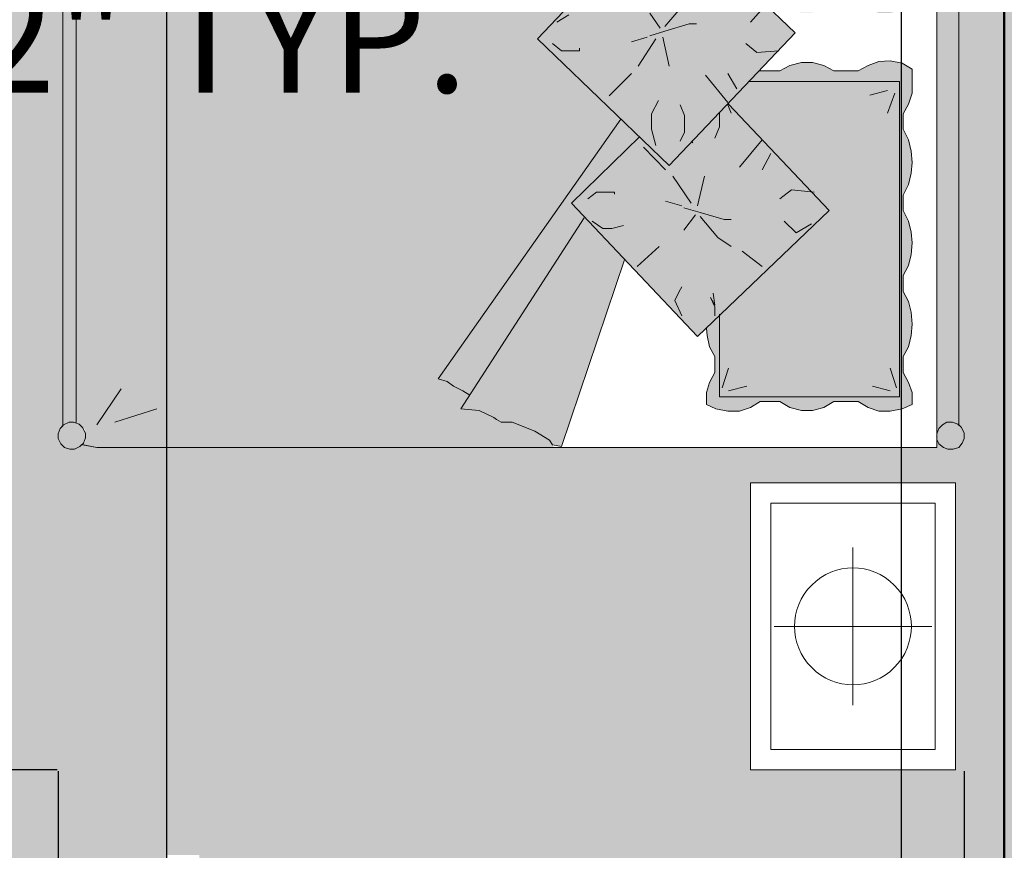
# Model space of a CAD drawing. Units: inches. Extents: x 528 to 2620, y -1066 to 798.
# Tile 28 of 41: x 1157 to 1211, y 620 to 665. Entities that reach past the tile are written whole.
import ezdxf

# ---------------------------------------------------------------- set-up
doc = ezdxf.new("R2010")
doc.units = ezdxf.units.IN
doc.header["$MEASUREMENT"] = 0
for name, color, linetype, lineweight in [('A-ANNO-DIMS', 2, 'Continuous', 18), ('A-FURN', 30, 'Continuous', 18), ('A-WALL', 7, 'Continuous', 50), ('A-WALL-PATT', 8, 'Continuous', 13)]:
    doc.layers.add(name, color=color, linetype=linetype, lineweight=lineweight)
doc.styles.get("Standard").update_dxf_attribs({"font": 'arial.ttf'})
doc.dimstyles.get("Standard").update_dxf_attribs({"dimtxt": 6, "dimasz": 2, "dimexe": 0.18, "dimexo": 0.0625, "dimgap": 0.09, "dimtad": 0, "dimtih": 1, "dimtoh": 1, "dimdec": 1, "dimzin": 0, "dimdsep": 46, "dimlunit": 3, "dimtxsty": 'Standard', "dimblk": 'ARCHTICK', "dimcen": 0.09, "dimadec": 0, "dimazin": 0, "dimtfac": 1, "dimtdec": 1, "dimtofl": 0, "dimtmove": 0, "dimatfit": 3, "dimfxl": 1, "dimtolj": 1, "dimtzin": 0, "dimarcsym": 0})

# ---------------------------------------------------------------- blocks, each defined once
blk = doc.blocks.new('d-bed-3')
at = {"color": 0, "linetype": 'ByBlock'}
for p, q in [((0.8389, 0.0078), (2.7305, 0.0078)), ((0.8409, 0.0078), (2.7305, 0.0078)), ((2.7234, -0.0077), (2.7284, 0.0056)), ((2.7284, 0.0056), (2.7365, 0.0144)), ((2.7305, 0.0078), (2.7365, 0.0144)), ((2.7365, 0.0144), (2.7505, 0.0211)), ((2.7365, 0.0144), (2.7505, 0.0211)), ((2.7505, 0.0211), (2.7636, 0.0211)), ((2.7505, 0.0211), (2.7636, 0.0211)), ((2.7636, 0.0211), (2.7746, 0.0166)), ((2.7636, 0.0211), (2.7746, 0.0166)), ((2.7746, 0.0166), (2.7857, 0.0078)), ((2.7746, 0.0166), (2.7857, 0.0078)), ((2.7857, 0.0078), (2.7897, -0.0054)), ((2.7857, 0.0078), (2.7897, -0.0054)), ((2.8714, -0.5), (2.8714, 0)), ((2.8714, 0), (3.5714, 0)), ((3.5714, 0), (3.5714, -0.5)), ((2.7234, -0.0209), (2.7234, -0.0077)), ((2.7305, -0.032), (2.7234, -0.0209)), ((2.7897, -0.0187), (2.7857, -0.0297)), ((2.7897, -0.0187), (2.7857, -0.0297)), ((2.7897, -0.0054), (2.7897, -0.0187)), ((2.7897, -0.0054), (2.7897, -0.0187)), ((2.7525, -0.0452), (0.8188, -0.0452)), ((2.7395, -0.0408), (2.7305, -0.032)), ((2.7525, -0.0452), (2.7395, -0.0408)), ((2.7656, -0.0452), (2.7525, -0.0452)), ((2.7766, -0.0408), (2.7656, -0.0452)), ((2.7766, -0.0408), (2.7656, -0.0452)), ((2.7656, -0.0452), (2.7857, -0.0452)), ((2.7857, -0.0452), (2.7656, -0.0452)), ((2.7857, -0.0297), (2.7766, -0.0408)), ((2.7857, -0.0297), (2.7766, -0.0408)), ((2.7857, -2.0939), (2.7857, -0.0452)), ((2.9214, -0.45), (2.9214, -0.05)), ((2.9214, -0.05), (3.5214, -0.05)), ((3.2214, -0.0576), (3.2214, -0.4424)), ((3.5214, -0.05), (3.5214, -0.45)), ((1.8489, -0.1302), (1.863, -0.1059)), ((1.863, -0.1059), (1.8951, -0.1059)), ((1.8951, -0.1059), (1.9222, -0.1059)), ((1.9222, -0.1059), (1.9483, -0.1148)), ((1.9483, -0.1148), (1.9724, -0.128)), ((2.0096, -0.128), (2.0357, -0.1148)), ((2.0357, -0.1148), (2.0628, -0.1082)), ((2.0628, -0.1082), (2.0909, -0.1059)), ((2.0909, -0.1059), (2.117, -0.1082)), ((2.117, -0.1082), (2.1441, -0.1148)), ((2.1441, -0.1148), (2.1702, -0.128)), ((2.2074, -0.128), (2.2335, -0.1148)), ((2.2335, -0.1148), (2.2606, -0.1082)), ((2.2606, -0.1082), (2.2867, -0.1059)), ((2.2867, -0.1059), (2.3148, -0.1082)), ((2.3148, -0.1082), (2.3419, -0.1148)), ((2.3419, -0.1148), (2.366, -0.128)), ((2.4052, -0.128), (2.4293, -0.1148)), ((2.4293, -0.1148), (2.4554, -0.1082)), ((2.4554, -0.1082), (2.4845, -0.1059)), ((2.4845, -0.1059), (2.5126, -0.1082)), ((2.5126, -0.1082), (2.5397, -0.1148)), ((2.5397, -0.1148), (2.5638, -0.128)), ((2.6029, -0.128), (2.627, -0.1148)), ((2.627, -0.1148), (2.6511, -0.1059)), ((2.6511, -0.1059), (2.6803, -0.1059)), ((2.6803, -0.1059), (2.6913, -0.1302)), ((1.8429, -0.159), (1.8489, -0.1302)), ((2.6622, -0.1369), (1.8931, -0.1369)), ((1.8931, -0.1369), (1.8931, -0.5046)), ((1.9724, -0.128), (2.0096, -0.128)), ((2.1702, -0.128), (2.2074, -0.128)), ((2.366, -0.128), (2.4052, -0.128)), ((2.5638, -0.128), (2.6029, -0.128)), ((2.6401, -0.1435), (2.5919, -0.159)), ((2.6622, -0.5753), (2.6622, -0.1369)), ((2.6913, -0.1302), (2.6973, -0.159)), ((1.8449, -0.1866), (1.8429, -0.159)), ((1.9152, -0.1656), (1.9263, -0.2087)), ((1.9222, -0.1479), (1.9704, -0.1656)), ((2.6471, -0.159), (2.6361, -0.202)), ((2.6973, -0.159), (2.6973, -0.1866)), ((1.854, -0.2131), (1.8449, -0.1866)), ((2.6973, -0.1866), (2.6883, -0.2131)), ((1.867, -0.2374), (1.854, -0.2131)), ((2.6883, -0.2131), (2.6732, -0.2374)), ((1.867, -0.297), (1.867, -0.2374)), ((2.6732, -0.2374), (2.6732, -0.297)), ((3.4138, -0.25), (3.029, -0.25)), ((1.854, -0.3213), (1.867, -0.297)), ((2.2074, -0.3081), (1.9483, -0.5532)), ((2.5146, -0.6294), (2.2074, -0.3081)), ((2.6732, -0.297), (2.6883, -0.3213)), ((1.8469, -0.3489), (1.854, -0.3213)), ((2.6883, -0.3213), (2.6953, -0.3489)), ((1.8469, -0.3754), (1.8469, -0.3489)), ((2.1632, -0.3445), (2.1572, -0.3997)), ((2.2405, -0.3511), (2.2626, -0.3887)), ((2.6953, -0.3489), (2.6953, -0.3754)), ((1.854, -0.4041), (1.8469, -0.3754)), ((2.6953, -0.3754), (2.6883, -0.4041)), ((1.4674, -0.7134), (1.7746, -0.3909)), ((1.7746, -0.3909), (2.0979, -0.6979)), ((1.867, -0.4284), (1.854, -0.4041)), ((2.1572, -0.3997), (2.1793, -0.4284)), ((2.2626, -0.3887), (2.2335, -0.4174)), ((2.6883, -0.4041), (2.6732, -0.4284)), ((1.8188, -0.4306), (1.8228, -0.4848)), ((1.867, -0.4781), (1.867, -0.4284)), ((2.6732, -0.4284), (2.6732, -0.4759)), ((2.0688, -0.4505), (2.109, -0.4715)), ((3.5214, -0.45), (2.9214, -0.45)), ((1.7194, -0.4737), (1.7485, -0.5002)), ((2.0357, -0.4715), (2.102, -0.5267)), ((2.3439, -0.4715), (2.3068, -0.5201)), ((2.6732, -0.4759), (2.6883, -0.5002)), ((1.8228, -0.4848), (1.8008, -0.5113)), ((2.6883, -0.5002), (2.6973, -0.5267)), ((3.5714, -0.5), (2.8714, -0.5)), ((2.6471, -0.5532), (2.6361, -0.5091)), ((2.6973, -0.5267), (2.6973, -0.5554)), ((1.9112, -0.5333), (1.874, -0.5554)), ((1.9704, -0.5466), (1.9503, -0.5554)), ((2.2295, -0.5643), (2.2295, -0.5466)), ((2.2736, -0.5797), (2.2957, -0.5466)), ((1.9443, -0.5554), (1.8781, -0.6096)), ((1.9684, -0.5753), (2.0036, -0.5753)), ((2.0036, -0.5753), (2.0317, -0.5864)), ((2.2124, -0.6228), (2.2295, -0.5643)), ((2.4604, -0.5753), (2.6622, -0.5753)), ((2.6401, -0.5687), (2.5919, -0.5532)), ((2.6973, -0.5554), (2.6913, -0.5841)), ((2.2224, -0.6228), (2.2736, -0.5797)), ((2.4383, -0.5864), (2.4092, -0.5908)), ((2.4423, -0.5864), (2.4202, -0.5974)), ((2.4202, -0.5974), (2.4383, -0.5864)), ((2.4644, -0.5864), (2.4423, -0.5864)), ((2.5397, -0.5996), (2.5126, -0.6051)), ((2.5638, -0.5864), (2.5397, -0.5996)), ((2.6029, -0.5864), (2.5638, -0.5864)), ((2.627, -0.5996), (2.6029, -0.5864)), ((2.6511, -0.6073), (2.627, -0.5996)), ((2.6913, -0.5841), (2.6803, -0.6073)), ((2.1963, -0.6294), (2.124, -0.6118)), ((2.2013, -0.6626), (2.2124, -0.6228)), ((2.5126, -0.6051), (2.4955, -0.6073)), ((2.6803, -0.6073), (2.6511, -0.6073)), ((1.7526, -0.6493), (1.7526, -0.6316)), ((2.0387, -0.6427), (2.0427, -0.6405)), ((2.1903, -0.6449), (2.124, -0.6891)), ((2.1903, -0.9365), (2.5146, -0.6294)), ((2.2556, -0.6626), (2.2184, -0.6338)), ((1.7596, -0.7089), (1.7084, -0.6648)), ((1.7706, -0.7089), (1.7526, -0.6493)), ((1.9765, -0.6604), (1.9503, -0.6714)), ((2.0166, -0.6604), (1.9765, -0.6604)), ((2.0387, -0.6714), (2.0166, -0.6604)), ((2.1963, -0.667), (2.1853, -0.7067)), ((2.4052, -0.6736), (2.3941, -0.667)), ((2.4644, -0.667), (2.4272, -0.6846)), ((2.4272, -0.6846), (2.4052, -0.6736)), ((1.7897, -1.0193), (1.4674, -0.7134)), ((1.7265, -0.7454), (1.7636, -0.72)), ((1.7817, -0.7454), (1.7706, -0.7089)), ((1.7857, -0.7134), (1.856, -0.6979)), ((2.0979, -0.6979), (1.7897, -1.0193)), ((2.0538, -0.7609), (2.109, -0.7067)), ((1.7897, -0.731), (1.856, -0.7741)), ((1.9724, -0.741), (1.9393, -0.7244)), ((2.0096, -0.741), (1.9724, -0.741)), ((2.0497, -0.731), (2.0096, -0.741)), ((2.3439, -0.7763), (2.2957, -0.7222)), ((1.7857, -0.752), (1.7967, -0.7896)), ((1.9283, -0.8448), (1.874, -0.7896)), ((2.1903, -0.9365), (2.0277, -0.7697)), ((2.618, -1.2611), (1.9855, -0.8161)), ((2.2515, -0.8382), (2.2445, -0.8094)), ((2.7827, -0.9607), (2.3278, -0.8072)), ((2.1632, -0.8757), (2.1632, -0.8315)), ((2.1632, -0.8315), (2.1682, -0.8315)), ((2.2515, -0.8602), (2.2515, -0.8382)), ((2.2335, -0.8856), (2.2515, -0.8602)), ((2.1793, -0.8967), (2.1632, -0.8757)), ((2.6913, -1.2059), (2.2254, -0.9055)), ((1.8188, -0.9166), (1.8118, -0.9166)), ((1.8188, -0.9607), (1.8188, -0.9166)), ((1.7485, -0.9718), (1.7305, -0.9431)), ((1.8008, -0.9828), (1.8188, -0.9607)), ((2.7786, -0.9828), (2.7676, -0.9895)), ((2.7827, -0.9607), (2.7786, -0.9828)), ((2.7676, -0.9895), (2.7455, -1.0259)), ((2.7455, -1.0259), (2.7234, -1.0811)), ((2.7234, -1.0811), (2.7234, -1.1076)), ((2.7124, -1.1253), (2.6953, -1.1617)), ((2.7174, -1.1187), (2.7124, -1.1253)), ((2.7234, -1.1076), (2.7174, -1.1187)), ((2.6953, -1.1617), (2.6913, -1.2059)), ((2.6582, -1.1838), (2.6471, -1.2015)), ((2.6361, -1.2236), (2.625, -1.2391)), ((2.6471, -1.2015), (2.6361, -1.2236)), ((2.625, -1.2391), (2.618, -1.2611)), ((2.7234, -2.0497), (2.6913, -1.947)), ((2.7305, -2.0939), (2.6421, -2.0342)), ((2.7857, -2.0939), (2.7783, -2.1299)), ((2.7786, -2.1281), (2.7857, -2.0939)), ((2.7365, -2.1281), (2.7284, -2.1369)), ((2.7505, -2.1215), (2.7365, -2.1281)), ((2.7616, -2.1215), (2.7505, -2.1215)), ((2.7746, -2.1259), (2.7616, -2.1215)), ((2.7827, -2.1347), (2.7746, -2.1259)), ((2.7783, -2.1299), (2.7827, -2.1347)), ((2.7827, -2.1347), (2.7897, -2.148)), ((2.7897, -2.148), (2.7827, -2.1347)), ((2.7264, -2.1436), (0.845, -2.1436)), ((2.7284, -2.1369), (2.7234, -2.1502)), ((2.7234, -2.1502), (2.7234, -2.1612)), ((2.7897, -2.159), (2.7857, -2.1723)), ((2.7857, -2.1723), (2.7897, -2.159)), ((2.7897, -2.148), (2.7897, -2.159)), ((2.7897, -2.159), (2.7897, -2.148)), ((2.7327, -2.1767), (0.8367, -2.1767)), ((0.8389, -2.1767), (2.7305, -2.1767)), ((2.7234, -2.1612), (2.7305, -2.1745)), ((2.7305, -2.1745), (2.7395, -2.1833)), ((2.7395, -2.1833), (2.7327, -2.1767)), ((2.7525, -2.1877), (2.7395, -2.1833)), ((2.7395, -2.1833), (2.7525, -2.1877)), ((2.7766, -2.1811), (2.7636, -2.1877)), ((2.7636, -2.1877), (2.7766, -2.1811)), ((2.7857, -2.1723), (2.7766, -2.1811)), ((2.7766, -2.1811), (2.7857, -2.1723)), ((2.7636, -2.1877), (2.7525, -2.1877)), ((2.7525, -2.1877), (2.7636, -2.1877))]:
    blk.add_line(p, q, dxfattribs=at)
at = {"color": 0, "linetype": 'ByBlock', "extrusion": (0, 0, -1)}
blk.add_ellipse((3.2214, -0.25), major_axis=(0.1007, 0.1007), ratio=1, dxfattribs=at)
blk = doc.blocks.new('_ArchTick')
at = {"color": 0, "linetype": 'ByBlock', "const_width": 0.15}
blk.add_lwpolyline([(-0.5, -0.5), (0.5, 0.5)], dxfattribs=at)
blk = doc.blocks.new('*D42')
at = {"layer": 'A-ANNO-DIMS', "color": 0, "lineweight": -2, "transparency": 16777216}
for p, q in [((1159.521, 703.64), (1147.464, 703.64)), ((1147.644, 703.64), (1147.644, 667.032)), ((1147.644, 624.039), (1147.644, 660.647)), ((1159.521, 624.039), (1147.464, 624.039))]:
    blk.add_line(p, q, dxfattribs=at)
at = {"layer": 'Defpoints', "color": 0, "transparency": 16777216}
for p in [(1159.584, 703.64), (1147.644, 624.039), (1159.584, 624.039)]:
    blk.add_point(p, dxfattribs=at)
at = {"layer": 'A-ANNO-DIMS', "color": 0, "lineweight": -2, "transparency": 16777216, "xscale": 2, "yscale": 2, "zscale": 2}
for p, rotation in [((1147.644, 703.64), 90), ((1147.644, 624.039), 270)]:
    blk.add_blockref('_ArchTick', p, dxfattribs=dict(at, rotation=rotation))
at = {"layer": 'A-ANNO-DIMS', "color": 0, "transparency": 16777216, "insert": (1147.644, 663.839), "char_height": 6, "attachment_point": 5}
blk.add_mtext('\\A1;BED 6\'-7 1/2" TYP.', dxfattribs=at)
blk = doc.blocks.new('*D43')
at = {"layer": 'A-ANNO-DIMS', "color": 0, "lineweight": -2, "transparency": 16777216}
for p, q in [((1159.584, 623.976), (1159.584, 611.919)), ((1208.815, 623.976), (1208.815, 611.919)), ((1159.584, 612.099), (1165.702, 612.099)), ((1208.815, 612.099), (1202.696, 612.099))]:
    blk.add_line(p, q, dxfattribs=at)
at = {"layer": 'Defpoints', "color": 0, "transparency": 16777216}
for p in [(1159.584, 624.039), (1208.815, 624.039), (1208.815, 612.099)]:
    blk.add_point(p, dxfattribs=at)
at = {"layer": 'A-ANNO-DIMS', "color": 0, "lineweight": -2, "transparency": 16777216, "xscale": 2, "yscale": 2, "zscale": 2, "rotation": 180}
blk.add_blockref('_ArchTick', (1159.584, 612.099), dxfattribs=at)
at = {"layer": 'A-ANNO-DIMS', "color": 0, "lineweight": -2, "transparency": 16777216, "xscale": 2, "yscale": 2, "zscale": 2}
blk.add_blockref('_ArchTick', (1208.815, 612.099), dxfattribs=at)
at = {"layer": 'A-ANNO-DIMS', "color": 0, "transparency": 16777216, "insert": (1184.199, 612.099), "char_height": 6, "attachment_point": 5}
blk.add_mtext('\\A1;4\'-1" TYP.', dxfattribs=at)
blk = doc.blocks.new('*D58')
at = {"layer": 'A-ANNO-DIMS', "color": 0, "lineweight": -2, "transparency": 16777216}
for p, q in [((1165.496, 577.985), (1165.496, 751.102)), ((1165.496, 750.922), (1177.395, 750.922)), ((1205.418, 750.922), (1193.52, 750.922)), ((1205.418, 577.985), (1205.418, 751.102))]:
    blk.add_line(p, q, dxfattribs=at)
at = {"layer": 'Defpoints', "color": 0, "transparency": 16777216}
for p in [(1205.418, 750.922), (1165.496, 577.922), (1205.418, 577.922)]:
    blk.add_point(p, dxfattribs=at)
at = {"layer": 'A-ANNO-DIMS', "color": 0, "lineweight": -2, "transparency": 16777216, "xscale": 2, "yscale": 2, "zscale": 2, "rotation": 180}
blk.add_blockref('_ArchTick', (1165.496, 750.922), dxfattribs=at)
at = {"layer": 'A-ANNO-DIMS', "color": 0, "lineweight": -2, "transparency": 16777216, "xscale": 2, "yscale": 2, "zscale": 2}
blk.add_blockref('_ArchTick', (1205.418, 750.922), dxfattribs=at)
at = {"layer": 'A-ANNO-DIMS', "color": 0, "transparency": 16777216, "insert": (1185.457, 750.922), "char_height": 6, "attachment_point": 5}
blk.add_mtext('\\A1;3\'-4"', dxfattribs=at)

msp = doc.modelspace()

# ---------------------------------------------------------------- hatches: boundary and pattern name
at = {"layer": 'A-WALL-PATT', "transparency": 33554521}
h = msp.add_hatch(color=256, dxfattribs=at)
h.dxf.hatch_style = 1
h.paths.add_polyline_path([(1065.996, 709.922), (1114.496, 709.922), (1114.496, 718.922), (1056.996, 718.922), (1056.996, 667.922), (1065.996, 667.922)])
h.paths.add_polyline_path([(1227.496, 718.922), (1162.496, 718.922), (1162.496, 709.922), (1210.996, 709.922), (1210.996, 577.922), (1205.418, 577.922), (1205.496, 573.422), (1210.996, 573.422), (1210.996, 567.422), (1215.496, 567.422), (1215.496, 669.422), (1267.996, 669.422), (1267.996, 675.922), (1263.496, 675.922), (1263.496, 673.922), (1215.496, 673.922), (1215.496, 709.922), (1227.496, 709.922)])
h.paths.add_polyline_path([(1344.996, 718.922), (1315.996, 718.922), (1315.996, 709.922), (1335.996, 709.922), (1335.996, 641.672), (1344.996, 641.672)])
h.paths.add_polyline_path([(1065.996, 619.922), (1056.996, 619.922), (1056.996, 561.422), (1065.996, 561.422), (1065.996, 573.422), (1160.996, 573.422), (1160.996, 569.422), (1165.496, 569.422), (1165.496, 577.922), (1065.996, 577.922)])
h.paths.add_polyline_path([(1215.996, 391.422), (1215.996, 400.422), (1206.996, 400.422), (1200.996, 400.422), (1200.996, 397.422), (1200.996, 391.422), (1206.996, 391.422), (1206.996, 268.922), (1251.996, 268.922), (1251.996, 277.922), (1215.996, 277.922), (1215.996, 359.767)])
h.paths.add_polyline_path([(1344.996, 395.922), (1335.996, 395.922), (1287.996, 395.922), (1287.996, 391.422), (1335.996, 391.422), (1335.996, 277.922), (1299.996, 277.922), (1299.996, 268.922), (1344.996, 268.922)])
h.paths.add_polyline_path([(1344.996, 593.672), (1335.996, 593.672), (1335.996, 525.422), (1215.496, 525.422), (1215.496, 527.172), (1210.996, 527.172), (1210.996, 520.922), (1335.996, 520.922), (1335.996, 443.922), (1344.996, 443.922)])
h.paths.add_polyline_path([(1065.996, 520.922), (1165.496, 520.922), (1165.496, 545.422), (1160.996, 545.422), (1160.996, 525.422), (1065.996, 525.422), (1065.996, 537.422), (1056.996, 537.422), (1056.996, 484.672), (1065.996, 484.672)])
h.paths.add_polyline_path([(1065.996, 436.672), (1056.996, 436.672), (1056.996, 391.422), (1085.496, 391.422), (1085.496, 400.422), (1065.996, 400.422)])
h.paths.add_polyline_path([(1152.996, 397.422), (1152.996, 400.422), (1133.496, 400.422), (1133.496, 391.422), (1152.996, 391.422)])
at = {"layer": 'A-WALL-PATT', "transparency": 33554536}
h = msp.add_hatch(color=256, dxfattribs=at)
h.dxf.hatch_style = 1
h.paths.add_polyline_path([(1335.996, 709.922), (1267.996, 709.922), (1267.996, 699.922), (1266.746, 699.922), (1266.746, 675.922), (1267.996, 675.922), (1267.996, 669.422), (1215.496, 669.422), (1215.496, 567.172), (1216.996, 567.172), (1256.996, 567.172), (1256.996, 565.422), (1256.958, 565.422, -0.401453), (1216.996, 527.172), (1215.496, 527.172), (1215.496, 525.422), (1335.996, 525.422)], flags=17)
h.paths.add_polyline_path([(1285.032, 635.927), (1285.229, 636.128), (1285.672, 636.263), (1286.206, 636.02), (1286.976, 636.084), (1332.983, 636.084), (1333.363, 636.222), (1333.82, 636.084), (1334.115, 635.714), (1334.115, 635.3), (1333.907, 634.86), (1333.82, 634.827), (1333.82, 592.738), (1333.967, 592.604), (1334.115, 592.291), (1334.115, 591.877), (1333.82, 591.507), (1333.363, 591.369), (1332.983, 591.507), (1332.638, 591.789), (1332.638, 591.507), (1286.976, 591.507), (1286.173, 591.672), (1286.066, 591.574), (1285.681, 591.37), (1285.229, 591.507), (1285.032, 591.709), (1284.834, 592.098), (1284.983, 592.537), (1285.13, 592.688), (1285.13, 634.948), (1284.983, 635.099), (1284.834, 635.537)], flags=16)
h.paths.add_polyline_path([(1285.032, 635.927), (1285.229, 636.128), (1285.672, 636.263), (1286.206, 636.02), (1286.976, 636.084), (1332.983, 636.084), (1333.363, 636.222), (1333.82, 636.084), (1334.115, 635.714), (1334.115, 635.3), (1333.967, 634.987), (1333.82, 634.853), (1333.82, 592.738), (1333.967, 592.604), (1334.115, 592.291), (1334.115, 591.877), (1333.82, 591.507), (1333.363, 591.369), (1332.983, 591.507), (1332.638, 591.789), (1332.638, 592.246), (1332.638, 635.345), (1332.638, 635.802), (1332.983, 636.084), (1312.232, 636.084), (1311.1, 635.479), (1310.632, 635.479), (1310.435, 635.233), (1309.943, 635.099), (1309.696, 634.987), (1309.056, 634.763), (1308.712, 634.607), (1308.318, 634.607), (1307.752, 634.36), (1307.112, 634.271), (1307.013, 634.114), (1306.767, 634.025), (1307.255, 633.283), (1306.866, 633.04), (1306.767, 632.884), (1306.373, 632.637), (1306.029, 632.548), (1305.536, 632.414), (1315.472, 618.494), (1316.321, 619.388), (1312.773, 622.858), (1319.616, 630.109), (1320.067, 629.676), (1320.109, 629.997), (1320.281, 630.601), (1320.527, 631.183), (1320.527, 632.011), (1320.256, 632.548), (1320.109, 633.13), (1320.06, 633.734), (1320.626, 634.025), (1321.216, 634.159), (1321.856, 634.114), (1322.447, 633.913), (1322.989, 633.622), (1324.096, 633.622), (1324.638, 633.913), (1325.229, 634.07), (1325.869, 634.07), (1326.435, 633.913), (1326.976, 633.622), (1328.355, 633.622), (1328.896, 633.913), (1329.487, 634.114), (1330.103, 634.159), (1330.693, 634.025), (1331.284, 633.734), (1331.235, 633.13), (1331.087, 632.548), (1330.792, 632.011), (1330.792, 631.183), (1331.038, 630.601), (1331.235, 629.997), (1331.284, 629.415), (1331.186, 628.788), (1331.038, 628.184), (1330.792, 627.602), (1330.792, 626.774), (1331.038, 626.193), (1331.235, 625.588), (1331.284, 625.007), (1331.186, 624.38), (1331.038, 623.776), (1330.792, 623.239), (1330.792, 622.366), (1331.038, 621.829), (1331.235, 621.247), (1331.284, 620.598), (1331.186, 619.972), (1331.038, 619.367), (1330.792, 618.83), (1330.792, 617.958), (1331.087, 617.421), (1331.235, 616.884), (1331.284, 616.235), (1331.284, 615.518), (1330.693, 615.272), (1330.103, 615.116), (1329.487, 615.116), (1328.896, 615.317), (1328.355, 615.653), (1326.976, 615.653), (1326.435, 615.317), (1325.869, 615.16), (1325.229, 615.16), (1324.638, 615.317), (1324.096, 615.653), (1323.242, 615.653), (1324.933, 614.042), (1322.978, 611.983), (1324.096, 611.983), (1324.638, 612.274), (1325.278, 612.43), (1325.869, 612.43), (1326.484, 612.274), (1327.026, 611.983), (1328.355, 611.983), (1328.896, 612.274), (1329.487, 612.475), (1330.103, 612.52), (1330.743, 612.386), (1331.284, 612.072), (1331.284, 611.356), (1331.284, 610.752), (1331.087, 610.17), (1330.792, 609.633), (1330.792, 608.805), (1331.087, 608.223), (1331.235, 607.619), (1331.284, 606.993), (1331.235, 606.411), (1331.087, 605.807), (1330.792, 605.225), (1330.792, 604.397), (1331.087, 603.815), (1331.235, 603.211), (1331.284, 602.629), (1331.235, 602.002), (1331.087, 601.398), (1330.792, 600.861), (1330.792, 599.988), (1331.087, 599.451), (1331.235, 598.87), (1331.284, 598.221), (1331.235, 597.594), (1331.087, 596.99), (1330.792, 596.453), (1330.792, 595.58), (1331.087, 595.043), (1331.284, 594.506), (1331.284, 593.857), (1330.743, 593.611), (1330.103, 593.477), (1329.487, 593.477), (1328.896, 593.678), (1328.355, 594.014), (1327.026, 594.014), (1326.484, 593.678), (1325.869, 593.521), (1325.278, 593.521), (1324.638, 593.678), (1324.096, 594.014), (1323.038, 594.014), (1322.496, 593.678), (1321.906, 593.477), (1321.266, 593.477), (1320.626, 593.611), (1320.109, 593.857), (1320.109, 594.506), (1320.281, 595.043), (1320.576, 595.58), (1320.576, 596.453), (1320.281, 596.99), (1320.158, 597.594), (1320.104, 598.015), (1319.616, 597.549), (1315.659, 601.729), (1312.232, 591.574), (1311.74, 591.664), (1311.592, 591.91), (1310.78, 592.402), (1309.549, 592.895), (1308.958, 592.895), (1308.712, 593.029), (1308.564, 593.141), (1307.752, 593.521), (1306.767, 593.611), (1307.248, 594.356), (1306.866, 594.595), (1306.373, 594.842), (1306.029, 595.088), (1305.536, 595.244), (1315.465, 609.354), (1310.927, 613.706), (1315.472, 618.494), (1305.536, 632.414), (1306.029, 632.548), (1306.373, 632.637), (1306.767, 632.884), (1306.866, 633.04), (1307.255, 633.283), (1306.767, 634.025), (1307.013, 634.114), (1307.112, 634.271), (1307.752, 634.36), (1308.318, 634.607), (1308.712, 634.607), (1309.056, 634.763), (1309.696, 634.987), (1309.943, 635.099), (1310.435, 635.233), (1310.632, 635.479), (1311.1, 635.479), (1312.232, 636.084), (1286.976, 636.084), (1286.216, 636.021), (1286.411, 635.444), (1286.213, 635.054), (1286.016, 634.853), (1285.869, 634.808), (1285.869, 592.839), (1286.153, 592.731), (1286.41, 592.188), (1286.231, 591.66), (1286.173, 591.672), (1286.066, 591.574), (1285.681, 591.37), (1285.229, 591.507), (1285.032, 591.709), (1284.834, 592.098), (1284.983, 592.537), (1285.13, 592.688), (1285.13, 634.948), (1284.983, 635.099), (1284.834, 635.537)], flags=0)
h.paths.add_polyline_path([(1322.501, 653.596), (1333.646, 653.596), (1333.646, 637.994), (1322.501, 637.994)], flags=16)
h.paths.add_polyline_path([(1323.616, 652.482), (1332.531, 652.482), (1332.531, 639.108), (1323.616, 639.108)], flags=0)
edge = h.paths.add_edge_path(flags=0)
edge.add_ellipse((1328.073, 645.795), major_axis=(2.245, 2.245), ratio=1, start_angle=405, end_angle=495, ccw=False)
edge.add_ellipse((1328.073, 645.795), major_axis=(2.245, 2.245), ratio=1, start_angle=675, end_angle=765, ccw=False)
edge.add_ellipse((1328.073, 645.795), major_axis=(2.245, 2.245), ratio=1, start_angle=585, end_angle=675, ccw=False)
edge.add_ellipse((1328.073, 645.795), major_axis=(2.245, 2.245), ratio=1, start_angle=495, end_angle=585, ccw=False)
h.paths.add_polyline_path([(1320.576, 628.386), (1320.33, 628.005), (1320.615, 628.548)], flags=0)
h.paths.add_polyline_path([(1317.893, 604.889), (1318.78, 604.643), (1319.764, 604.285), (1318.878, 604.531)], flags=0)
h.paths.add_polyline_path([(1320.33, 599.653), (1320.576, 599.25), (1320.576, 599.16)], flags=0)
h.paths.add_polyline_path([(1322.501, 589.597), (1333.646, 589.597), (1333.646, 573.995), (1322.501, 573.995)], flags=16)
h.paths.add_polyline_path([(1323.616, 588.482), (1332.531, 588.482), (1332.531, 575.109), (1323.616, 575.109)], flags=0)
edge = h.paths.add_edge_path(flags=0)
edge.add_ellipse((1328.073, 581.796), major_axis=(-2.245, 2.245), ratio=1, start_angle=-45, end_angle=45, ccw=False)
edge.add_ellipse((1328.073, 581.796), major_axis=(-2.245, 2.245), ratio=1, start_angle=-135, end_angle=-45, ccw=False)
edge.add_ellipse((1328.073, 581.796), major_axis=(-2.245, 2.245), ratio=1, start_angle=135, end_angle=-135, ccw=False)
edge.add_ellipse((1328.073, 581.796), major_axis=(-2.245, 2.245), ratio=1, start_angle=45, end_angle=135, ccw=False)
h.paths.add_polyline_path([(1264.746, 699.922), (1263.496, 699.922), (1263.496, 709.922), (1215.496, 709.922), (1215.496, 673.922), (1263.496, 673.922), (1263.496, 675.922), (1264.746, 675.922)], flags=16)
h.paths.add_polyline_path([(1162.192, 569.422), (1160.996, 569.422), (1160.996, 573.422), (1065.996, 573.422), (1065.996, 525.422), (1160.996, 525.422), (1160.996, 545.422), (1162.192, 545.422)])
h.paths.add_polyline_path([(1256.958, 565.422), (1256.996, 565.422), (1256.996, 567.172), (1216.996, 567.172), (1215.496, 567.172), (1215.496, 567.422), (1210.996, 567.422), (1210.996, 573.422), (1205.496, 573.422), (1205.418, 577.922), (1210.996, 577.922), (1210.996, 709.922), (1065.996, 709.922), (1065.996, 577.922), (1165.496, 577.922), (1165.496, 569.422), (1164.192, 569.422), (1164.192, 545.422), (1165.496, 545.422), (1165.496, 520.922), (1152.996, 520.922), (1152.996, 484.922), (1101.996, 484.922), (1101.996, 436.422), (1152.996, 436.422), (1152.996, 400.422), (1152.996, 391.422), (1200.996, 391.422), (1200.996, 400.422), (1206.996, 400.422), (1215.996, 400.422), (1215.996, 391.422), (1215.996, 277.922), (1335.996, 277.922), (1335.996, 391.422), (1287.996, 391.422), (1287.996, 395.922), (1335.996, 395.922), (1335.996, 443.922), (1335.996, 520.922), (1210.996, 520.922), (1210.996, 527.172), (1215.496, 527.172), (1216.996, 527.172, 0.401453)])
h.paths.add_polyline_path([(1167.246, 579.422), (1165.496, 579.422), (1165.496, 619.422), (1167.246, 619.422)], flags=16)
h.paths.add_polyline_path([(1227.97, 501.564), (1236.36, 502.031), (1236.36, 492.555), (1227.97, 493.021, -0.254069)], flags=16)
h.paths.add_polyline_path([(1243.336, 515.692, -0.254069), (1251.879, 515.692), (1252.345, 507.301), (1242.87, 507.301)], flags=16)
h.paths.add_polyline_path([(1239.185, 504.685), (1256.03, 504.685), (1256.03, 479.416), (1239.185, 479.416)], flags=16)
h.paths.add_polyline_path([(1227.97, 489.602), (1236.36, 490.068), (1236.36, 480.592), (1227.97, 481.058, -0.254069)], flags=16)
h.paths.add_polyline_path([(1197.201, 624.039), (1197.201, 639.641), (1208.345, 639.641), (1208.345, 624.039)], flags=16)
h.paths.add_polyline_path([(1198.315, 625.153), (1198.315, 638.526), (1207.231, 638.526), (1207.231, 625.153)], flags=0)
h.paths.add_polyline_path([(1258.855, 502.031), (1267.245, 501.564, -0.254069), (1267.245, 493.021), (1258.855, 492.555)], flags=16)
h.paths.add_polyline_path([(1271.589, 519.657), (1333.671, 519.657), (1333.671, 451.595), (1319.087, 451.595), (1319.087, 505.072), (1288.093, 505.072), (1284.447, 505.072, -0.883215), (1270.678, 514.188), (1270.678, 518.745, -0.414214)], flags=16)
h.paths.add_polyline_path([(1331.848, 517.834), (1331.848, 453.418), (1328.202, 453.418), (1328.202, 505.072), (1298.424, 505.072), (1298.424, 514.188), (1288.093, 514.188), (1288.093, 517.834)], flags=0)
h.paths.add_polyline_path([(1242.87, 476.8), (1252.345, 476.8), (1251.879, 468.409, -0.254069), (1243.336, 468.409)], flags=16)
h.paths.add_polyline_path([(1258.855, 490.068), (1267.245, 489.602, -0.254069), (1267.245, 481.058), (1258.855, 480.592)], flags=16)
h.paths.add_polyline_path([(1161.676, 641.551), (1160.873, 641.716), (1160.765, 641.618), (1160.38, 641.414), (1159.928, 641.551), (1159.731, 641.753), (1159.534, 642.142), (1159.682, 642.581), (1159.83, 642.732), (1159.83, 684.992), (1159.682, 685.143), (1159.534, 685.582), (1159.731, 685.971), (1159.928, 686.172), (1160.371, 686.307), (1160.905, 686.064), (1161.676, 686.128), (1207.682, 686.128), (1208.063, 686.266), (1208.519, 686.128), (1208.815, 685.758), (1208.815, 685.344), (1208.607, 684.904), (1208.519, 684.871), (1208.519, 642.782), (1208.667, 642.648), (1208.877, 642.201), (1208.716, 641.797), (1208.519, 641.551), (1208.063, 641.413), (1207.682, 641.551), (1207.338, 641.833), (1207.338, 641.551)], flags=16)
h.paths.add_polyline_path([(1186.931, 641.618), (1186.439, 641.708), (1186.291, 641.954), (1185.479, 642.446), (1184.248, 642.939), (1183.658, 642.939), (1183.411, 643.073), (1183.264, 643.185), (1182.451, 643.565), (1181.467, 643.655), (1181.948, 644.4), (1181.565, 644.639), (1181.073, 644.886), (1180.728, 645.132), (1180.236, 645.288), (1190.164, 659.398), (1185.627, 663.75), (1190.171, 668.538), (1180.236, 682.458), (1180.728, 682.592), (1181.073, 682.681), (1181.467, 682.928), (1181.565, 683.084), (1181.954, 683.327), (1181.467, 684.069), (1181.713, 684.158), (1181.811, 684.315), (1182.451, 684.404), (1183.018, 684.651), (1183.411, 684.651), (1183.756, 684.807), (1184.396, 685.031), (1184.642, 685.143), (1185.135, 685.277), (1185.331, 685.523), (1185.799, 685.523), (1186.931, 686.128), (1161.676, 686.128), (1160.915, 686.065), (1161.111, 685.488), (1160.913, 685.098), (1160.716, 684.897), (1160.568, 684.852), (1160.568, 642.883), (1160.853, 642.775), (1161.109, 642.232), (1160.931, 641.704), (1160.873, 641.716), (1160.765, 641.618), (1160.38, 641.414), (1159.928, 641.551), (1159.731, 641.753), (1159.534, 642.142), (1159.682, 642.581), (1159.83, 642.732), (1159.83, 684.992), (1159.682, 685.143), (1159.534, 685.582), (1159.731, 685.971), (1159.928, 686.172), (1160.371, 686.307), (1160.905, 686.064), (1161.676, 686.128), (1207.682, 686.128), (1208.063, 686.266), (1208.519, 686.128), (1208.815, 685.758), (1208.815, 685.344), (1208.667, 685.031), (1208.519, 684.897), (1208.519, 642.782), (1208.667, 642.648), (1208.877, 642.201), (1208.716, 641.797), (1208.519, 641.551), (1208.063, 641.413), (1207.682, 641.551), (1207.338, 641.833), (1207.338, 642.29), (1207.338, 685.389), (1207.338, 685.846), (1207.682, 686.128), (1186.931, 686.128), (1185.799, 685.523), (1185.331, 685.523), (1185.135, 685.277), (1184.642, 685.143), (1184.396, 685.031), (1183.756, 684.807), (1183.411, 684.651), (1183.018, 684.651), (1182.451, 684.404), (1181.811, 684.315), (1181.713, 684.158), (1181.467, 684.069), (1181.954, 683.327), (1181.565, 683.084), (1181.467, 682.928), (1181.073, 682.681), (1180.728, 682.592), (1180.236, 682.458), (1190.171, 668.538), (1191.021, 669.432), (1187.473, 672.902), (1194.316, 680.153), (1194.767, 679.72), (1194.808, 680.041), (1194.981, 680.645), (1195.227, 681.227), (1195.227, 682.055), (1194.956, 682.592), (1194.808, 683.174), (1194.759, 683.778), (1195.325, 684.069), (1195.916, 684.203), (1196.556, 684.158), (1197.147, 683.957), (1197.688, 683.666), (1198.796, 683.666), (1199.338, 683.957), (1199.928, 684.114), (1200.568, 684.114), (1201.135, 683.957), (1201.676, 683.666), (1203.055, 683.666), (1203.596, 683.957), (1204.187, 684.158), (1204.802, 684.203), (1205.393, 684.069), (1205.984, 683.778), (1205.935, 683.174), (1205.787, 682.592), (1205.491, 682.055), (1205.491, 681.227), (1205.738, 680.645), (1205.935, 680.041), (1205.984, 679.459), (1205.885, 678.832), (1205.738, 678.228), (1205.491, 677.646), (1205.491, 676.818), (1205.738, 676.237), (1205.935, 675.632), (1205.984, 675.051), (1205.885, 674.424), (1205.738, 673.82), (1205.491, 673.283), (1205.491, 672.41), (1205.738, 671.873), (1205.935, 671.291), (1205.984, 670.642), (1205.885, 670.016), (1205.738, 669.411), (1205.491, 668.874), (1205.491, 668.002), (1205.787, 667.465), (1205.935, 666.928), (1205.984, 666.279), (1205.984, 665.563), (1205.393, 665.316), (1204.802, 665.16), (1204.187, 665.16), (1203.596, 665.361), (1203.055, 665.697), (1201.676, 665.697), (1201.135, 665.361), (1200.568, 665.204), (1199.928, 665.204), (1199.338, 665.361), (1198.796, 665.697), (1197.942, 665.697), (1199.633, 664.086), (1197.678, 662.027), (1198.796, 662.027), (1199.338, 662.318), (1199.978, 662.474), (1200.568, 662.474), (1201.184, 662.318), (1201.725, 662.027), (1203.055, 662.027), (1203.596, 662.318), (1204.187, 662.519), (1204.802, 662.564), (1205.442, 662.43), (1205.984, 662.116), (1205.984, 661.4), (1205.984, 660.796), (1205.787, 660.214), (1205.491, 659.677), (1205.491, 658.849), (1205.787, 658.267), (1205.935, 657.663), (1205.984, 657.037), (1205.935, 656.455), (1205.787, 655.851), (1205.491, 655.269), (1205.491, 654.441), (1205.787, 653.859), (1205.935, 653.255), (1205.984, 652.673), (1205.935, 652.046), (1205.787, 651.442), (1205.491, 650.905), (1205.491, 650.032), (1205.787, 649.495), (1205.935, 648.914), (1205.984, 648.265), (1205.935, 647.638), (1205.787, 647.034), (1205.491, 646.497), (1205.491, 645.624), (1205.787, 645.087), (1205.984, 644.55), (1205.984, 643.901), (1205.442, 643.655), (1204.802, 643.521), (1204.187, 643.521), (1203.596, 643.722), (1203.055, 644.058), (1201.725, 644.058), (1201.184, 643.722), (1200.568, 643.565), (1199.978, 643.565), (1199.338, 643.722), (1198.796, 644.058), (1197.738, 644.058), (1197.196, 643.722), (1196.605, 643.521), (1195.965, 643.521), (1195.325, 643.655), (1194.808, 643.901), (1194.808, 644.55), (1194.981, 645.087), (1195.276, 645.624), (1195.276, 646.497), (1194.981, 647.034), (1194.858, 647.638), (1194.803, 648.059), (1194.316, 647.593), (1190.359, 651.773)], flags=16)
h.paths.add_polyline_path([(1195.276, 649.204), (1195.03, 649.697), (1195.276, 649.294)], flags=0)
h.paths.add_polyline_path([(1194.464, 654.329), (1193.578, 654.575), (1192.593, 654.933), (1193.479, 654.687)], flags=0)
h.paths.add_polyline_path([(1195.276, 678.43), (1195.03, 678.049), (1195.314, 678.592)], flags=0)
h.paths.add_polyline_path([(1197.201, 688.038), (1197.201, 703.64), (1208.345, 703.64), (1208.345, 688.038)], flags=16)
h.paths.add_polyline_path([(1198.315, 689.152), (1198.315, 702.526), (1207.231, 702.526), (1207.231, 689.152)], flags=0)
h.paths.add_polyline_path([(1217.099, 329.02), (1230.651, 329.02), (1230.651, 315.468), (1217.099, 315.468)], flags=16)
h.paths.add_polyline_path([(1223.875, 322.244), (1227.263, 322.244), (1227.263, 321.322, -0.414214), (1229.729, 318.856, -1), (1224.797, 318.856), (1223.875, 318.856)], flags=0)
h.paths.add_polyline_path([(1222.115, 325.632, -1), (1218.859, 325.632, -1)], flags=0)
h.paths.add_polyline_path([(1228.25, 325.632, -1), (1226.276, 325.632, -1)], flags=0)
h.paths.add_polyline_path([(1221.533, 318.856, -1), (1219.441, 318.856, -1)], flags=0)
h.paths.add_polyline_path([(1299.145, 293.732), (1299.145, 278.539), (1271.232, 278.539), (1271.232, 293.732)], flags=16)
h.paths.add_polyline_path([(1259.687, 292.213), (1270.624, 292.213, -1), (1270.624, 291.605), (1259.687, 291.605, -1)], flags=16)
h.paths.add_polyline_path([(1259.687, 291.301), (1270.624, 291.301, -1), (1270.624, 290.693), (1259.687, 290.693, -1)], flags=16)
h.paths.add_polyline_path([(1259.687, 290.389), (1270.624, 290.389, -1), (1270.624, 289.782), (1259.687, 289.782, -1)], flags=16)
h.paths.add_polyline_path([(1259.687, 289.478), (1270.624, 289.478, -1), (1270.624, 288.87), (1259.687, 288.87, -1)], flags=16)
h.paths.add_polyline_path([(1259.687, 288.566), (1270.624, 288.566, -1), (1270.624, 287.958), (1259.687, 287.958, -1)], flags=16)
h.paths.add_polyline_path([(1274.406, 292.381), (1283.251, 292.381, -0.414214), (1285.074, 290.558), (1285.074, 283.642, -0.414214), (1283.251, 281.819), (1277.723, 281.819), (1278.673, 280.869, -0.57735), (1279.382, 280.16), (1279.436, 280.106, -1), (1279.027, 279.696), (1278.972, 279.751, -0.57735), (1278.263, 280.46), (1276.904, 281.819), (1274.406, 281.819, -0.414214), (1272.583, 283.642), (1272.583, 290.558, -0.414214)], flags=0)
h.paths.add_polyline_path([(1259.687, 287.655), (1270.624, 287.655, -1), (1270.624, 287.047), (1259.687, 287.047, -1)], flags=16)
h.paths.add_polyline_path([(1259.687, 286.743), (1270.624, 286.743, -1), (1270.624, 286.135), (1259.687, 286.135, -1)], flags=16)
h.paths.add_polyline_path([(1259.687, 285.831), (1270.624, 285.831, -1), (1270.624, 285.224), (1259.687, 285.224, -1)], flags=16)
h.paths.add_polyline_path([(1259.687, 284.92), (1270.624, 284.92, -1), (1270.624, 284.312), (1259.687, 284.312, -1)], flags=16)
h.paths.add_polyline_path([(1259.687, 284.008), (1270.624, 284.008, -1), (1270.624, 283.401), (1259.687, 283.401, -1)], flags=16)
h.paths.add_polyline_path([(1287.823, 292.381), (1296.669, 292.381, -0.414214), (1298.492, 290.558), (1298.492, 283.642, -0.414214), (1296.669, 281.819), (1291.14, 281.819), (1292.09, 280.869, -0.57735), (1292.799, 280.16), (1292.854, 280.106, -1), (1292.445, 279.696), (1292.39, 279.751, -0.57735), (1291.681, 280.46), (1290.322, 281.819), (1287.823, 281.819, -0.414214), (1286, 283.642), (1286, 290.558, -0.414214)], flags=0)
h.paths.add_polyline_path([(1259.687, 283.097), (1270.624, 283.097, -1), (1270.624, 282.489), (1259.687, 282.489, -1)], flags=16)
h.paths.add_polyline_path([(1279.939, 287.607, -1), (1278.01, 287.607, -1)], flags=0)
h.paths.add_polyline_path([(1259.687, 282.185), (1270.624, 282.185, -1), (1270.624, 281.577), (1259.687, 281.577, -1)], flags=16)
h.paths.add_polyline_path([(1259.687, 281.273), (1270.624, 281.273, -1), (1270.624, 280.666), (1259.687, 280.666, -1)], flags=16)
h.paths.add_polyline_path([(1275.156, 284.169, -1), (1274.77, 284.169, -1)], flags=0)
h.paths.add_polyline_path([(1293.357, 287.607, -1), (1291.427, 287.607, -1)], flags=0)
h.paths.add_polyline_path([(1275.144, 280.503), (1276.335, 280.503, -5.828427), (1276.335, 280.117), (1275.144, 280.117, -1)], flags=0)
h.paths.add_polyline_path([(1288.574, 284.169, -1), (1288.188, 284.169, -1)], flags=0)
h.paths.add_polyline_path([(1281.31, 280.503), (1282.501, 280.503, -1), (1282.501, 280.117), (1281.31, 280.117, -5.828427)], flags=0)
h.paths.add_polyline_path([(1288.562, 280.503), (1289.752, 280.503, -5.828427), (1289.752, 280.117), (1288.562, 280.117, -1)], flags=0)
h.paths.add_polyline_path([(1294.727, 280.503), (1295.918, 280.503, -1), (1295.918, 280.117), (1294.727, 280.117, -5.828427)], flags=0)
h.paths.add_polyline_path([(1206.996, 391.422), (1200.996, 391.422), (1061.496, 391.422), (1061.496, 307.96), (1068.996, 307.96), (1068.996, 305.422), (1206.996, 305.422)])
at = {"layer": 'A-WALL-PATT', "transparency": 33554480}
h = msp.add_hatch(color=256, dxfattribs=at)
h.dxf.hatch_style = 1
h.paths.add_polyline_path([(1210.996, 709.922), (1065.996, 709.922), (1065.996, 577.922), (1165.496, 577.922), (1165.496, 579.422), (1165.496, 619.422), (1167.246, 619.422), (1167.246, 619.384, -0.401453), (1205.496, 579.422), (1205.496, 577.922), (1210.996, 577.922)])
h.paths.add_polyline_path([(1160.833, 686.058), (1160.905, 686.064), (1160.765, 686.128)], flags=16)
h.paths.add_polyline_path([(1160.931, 641.704), (1160.931, 641.707), (1160.928, 641.705)], flags=0)
h.paths.add_polyline_path([(1159.83, 684.992), (1159.584, 685.244), (1159.584, 685.82), (1160.016, 686.262), (1160.224, 686.262), (1159.928, 686.172), (1159.731, 685.971), (1159.584, 685.68), (1159.584, 685.434), (1159.682, 685.143), (1159.879, 684.942), (1160.175, 684.807), (1160.421, 684.807), (1160.716, 684.897), (1160.913, 685.098), (1161.111, 685.488), (1161.061, 685.635), (1161.061, 685.249), (1160.568, 684.746), (1160.568, 642.961), (1161.061, 642.514), (1161.061, 641.887), (1160.873, 641.716), (1161.676, 641.551), (1186.533, 641.551), (1186.291, 641.954), (1185.479, 642.446), (1184.248, 642.939), (1183.589, 642.939), (1183.264, 643.185), (1182.451, 643.565), (1181.467, 643.655), (1181.948, 644.4), (1181.565, 644.639), (1181.073, 644.886), (1180.728, 645.132), (1180.236, 645.288), (1190.164, 659.398), (1185.627, 663.75), (1190.171, 668.538), (1180.236, 682.458), (1180.728, 682.592), (1181.073, 682.681), (1181.467, 682.928), (1181.565, 683.084), (1181.954, 683.327), (1181.467, 684.069), (1181.713, 684.158), (1181.811, 684.315), (1182.451, 684.404), (1183.018, 684.651), (1183.411, 684.651), (1183.756, 684.807), (1184.396, 685.031), (1184.642, 685.143), (1185.135, 685.277), (1185.331, 685.523), (1185.799, 685.523), (1186.931, 686.128), (1207.682, 686.128), (1208.063, 686.266), (1208.631, 686.094), (1208.877, 685.478), (1208.607, 684.904), (1208.519, 684.871), (1208.519, 642.782), (1208.815, 642.514), (1208.815, 641.921), (1208.448, 641.462), (1207.792, 641.462), (1207.338, 641.833), (1207.338, 641.551), (1161.676, 641.551), (1160.928, 641.705), (1160.38, 641.414), (1159.816, 641.585), (1159.534, 642.142), (1159.722, 642.699), (1159.83, 642.756)], flags=16)
h.paths.add_polyline_path([(1159.83, 684.992), (1159.584, 685.244), (1159.584, 685.82), (1160.016, 686.262), (1160.224, 686.262), (1159.928, 686.172), (1159.731, 685.971), (1159.584, 685.68), (1159.584, 685.434), (1159.682, 685.143), (1159.83, 684.992), (1159.83, 642.732), (1159.682, 642.581), (1159.584, 642.29), (1159.584, 642.044), (1159.731, 641.753), (1160.016, 641.462), (1160.224, 641.462), (1159.816, 641.585), (1159.534, 642.142), (1159.682, 642.581), (1159.83, 642.732)], flags=0)
h.paths.add_polyline_path([(1207.682, 686.128), (1207.517, 686.128), (1207.488, 686.057)], flags=0)
h.paths.add_polyline_path([(1195.276, 648.712), (1195.287, 648.521), (1195.522, 648.746), (1195.522, 648.802), (1195.276, 649.204)], flags=0)
h.paths.add_polyline_path([(1194.767, 679.72), (1194.808, 680.041), (1194.981, 680.645), (1195.227, 681.227), (1195.227, 682.055), (1194.956, 682.592), (1194.808, 683.174), (1194.759, 683.778), (1195.325, 684.069), (1195.916, 684.203), (1196.556, 684.158), (1197.147, 683.957), (1197.688, 683.666), (1198.796, 683.666), (1199.338, 683.957), (1199.928, 684.114), (1200.568, 684.114), (1201.135, 683.957), (1201.676, 683.666), (1203.055, 683.666), (1203.596, 683.957), (1204.187, 684.158), (1204.802, 684.203), (1205.393, 684.069), (1205.984, 683.778), (1205.935, 683.174), (1205.787, 682.592), (1205.491, 682.055), (1205.491, 681.227), (1205.738, 680.645), (1205.935, 680.041), (1205.984, 679.459), (1205.885, 678.832), (1205.738, 678.228), (1205.491, 677.646), (1205.491, 676.818), (1205.738, 676.237), (1205.935, 675.632), (1205.984, 675.051), (1205.885, 674.424), (1205.738, 673.82), (1205.491, 673.283), (1205.491, 672.41), (1205.738, 671.873), (1205.935, 671.291), (1205.984, 670.642), (1205.885, 670.016), (1205.738, 669.411), (1205.491, 668.874), (1205.491, 668.002), (1205.787, 667.465), (1205.935, 666.928), (1205.984, 666.279), (1205.984, 665.563), (1205.393, 665.316), (1204.802, 665.16), (1204.187, 665.16), (1203.596, 665.361), (1203.055, 665.697), (1201.676, 665.697), (1201.135, 665.361), (1200.568, 665.204), (1199.928, 665.204), (1199.338, 665.361), (1198.796, 665.697), (1197.942, 665.697), (1199.633, 664.086), (1197.678, 662.027), (1198.796, 662.027), (1199.338, 662.318), (1199.978, 662.474), (1200.568, 662.474), (1201.184, 662.318), (1201.725, 662.027), (1203.055, 662.027), (1203.596, 662.318), (1204.187, 662.519), (1204.802, 662.564), (1205.442, 662.43), (1205.984, 662.116), (1205.984, 661.4), (1205.984, 660.796), (1205.787, 660.214), (1205.491, 659.677), (1205.491, 658.849), (1205.787, 658.267), (1205.935, 657.663), (1205.984, 657.037), (1205.935, 656.455), (1205.787, 655.851), (1205.491, 655.269), (1205.491, 654.441), (1205.787, 653.859), (1205.935, 653.255), (1205.984, 652.673), (1205.935, 652.046), (1205.787, 651.442), (1205.491, 650.905), (1205.491, 650.032), (1205.787, 649.495), (1205.935, 648.914), (1205.984, 648.265), (1205.935, 647.638), (1205.787, 647.034), (1205.491, 646.497), (1205.491, 645.624), (1205.787, 645.087), (1205.984, 644.55), (1205.984, 643.901), (1205.442, 643.655), (1204.802, 643.521), (1204.187, 643.521), (1203.596, 643.722), (1203.055, 644.058), (1201.725, 644.058), (1201.184, 643.722), (1200.568, 643.565), (1199.978, 643.565), (1199.338, 643.722), (1198.796, 644.058), (1197.738, 644.058), (1195.522, 644.304), (1205.295, 644.304), (1205.295, 661.445), (1197.125, 661.445), (1199.633, 664.086), (1196.004, 667.543), (1201.479, 673.283), (1195.522, 678.996), (1195.522, 678.922), (1195.31, 678.575), (1195.276, 678.43), (1195.03, 678.049), (1195.276, 678.519), (1195.276, 679.232)], flags=0)
h.paths.add_polyline_path([(1192.593, 654.933), (1193.479, 654.687), (1194.464, 654.329), (1193.578, 654.575)], flags=0)
h.paths.add_polyline_path([(1192.593, 672.79), (1193.43, 673.037), (1194.295, 673.351), (1194.29, 673.358), (1193.578, 673.149)], flags=0)
h.paths.add_polyline_path([(1195.276, 649.294), (1195.03, 649.697), (1195.296, 649.165)], flags=0)
h.paths.add_polyline_path([(1197.201, 639.641), (1208.345, 639.641), (1208.345, 624.039), (1197.201, 624.039)], flags=16)
h.paths.add_polyline_path([(1198.315, 638.526), (1207.231, 638.526), (1207.231, 625.153), (1198.315, 625.153)], flags=0)
edge = h.paths.add_edge_path(flags=0)
edge.add_ellipse((1202.773, 631.84), major_axis=(-2.245, 2.245), ratio=1, start_angle=-45, end_angle=45, ccw=False)
edge.add_ellipse((1202.773, 631.84), major_axis=(-2.245, 2.245), ratio=1, start_angle=-135, end_angle=-45, ccw=False)
edge.add_ellipse((1202.773, 631.84), major_axis=(-2.245, 2.245), ratio=1, start_angle=135, end_angle=-135, ccw=False)
edge.add_ellipse((1202.773, 631.84), major_axis=(-2.245, 2.245), ratio=1, start_angle=45, end_angle=135, ccw=False)
h.paths.add_polyline_path([(1197.201, 688.038), (1197.201, 703.64), (1208.345, 703.64), (1208.345, 688.038)], flags=16)
h.paths.add_polyline_path([(1198.315, 689.152), (1198.315, 702.526), (1207.231, 702.526), (1207.231, 689.152)], flags=0)
edge = h.paths.add_edge_path(flags=0)
edge.add_ellipse((1202.773, 695.839), major_axis=(2.245, 2.245), ratio=1, start_angle=405, end_angle=495, ccw=False)
edge.add_ellipse((1202.773, 695.839), major_axis=(2.245, 2.245), ratio=1, start_angle=675, end_angle=765, ccw=False)
edge.add_ellipse((1202.773, 695.839), major_axis=(2.245, 2.245), ratio=1, start_angle=585, end_angle=675, ccw=False)
edge.add_ellipse((1202.773, 695.839), major_axis=(2.245, 2.245), ratio=1, start_angle=495, end_angle=585, ccw=False)
h.paths.add_polyline_path([(1207.338, 685.389), (1207.338, 685.846), (1207.792, 686.217), (1208.448, 686.217), (1208.815, 685.758), (1208.815, 685.165), (1208.519, 684.897), (1208.519, 642.782), (1208.815, 642.514), (1208.815, 641.921), (1208.448, 641.462), (1207.792, 641.462), (1207.338, 641.833), (1207.338, 642.29)], flags=0)
h.paths.add_polyline_path([(1207.469, 642.678), (1207.989, 643.009), (1208.607, 642.775), (1208.877, 642.201), (1208.631, 641.585), (1208.063, 641.413), (1207.488, 641.622), (1207.284, 642.132)], flags=16)
h.paths.add_polyline_path([(1207.633, 684.897), (1207.879, 684.74), (1208.347, 684.74), (1208.667, 685.031), (1208.815, 685.344), (1208.815, 685.635), (1208.716, 685.881), (1208.448, 686.217), (1208.224, 686.217), (1208.631, 686.094), (1208.877, 685.478), (1208.667, 685.031), (1208.347, 684.74), (1207.786, 684.74)], flags=16)
h.paths.add_polyline_path([(1076.476, 648.31), (1137.071, 648.31), (1137.071, 658.865), (1076.476, 658.865)], flags=24)
h.paths.add_polyline_path([(1076.71, 662.103), (1130.014, 662.103), (1130.014, 672.798), (1076.71, 672.798)], flags=24)

# ---------------------------------------------------------------- linework, layer by layer
at = {"layer": 'A-WALL'}
msp.add_line((1210.996, 709.922), (1210.996, 577.922), dxfattribs=at)

# ---------------------------------------------------------------- block references
at = {"layer": 'A-FURN', "xscale": 22.28859121186505, "yscale": 22.28859121186505, "zscale": 22.28859121186505, "rotation": 270}
msp.add_blockref('d-bed-3', (1208.345, 703.64), dxfattribs=at)

# ---------------------------------------------------------------- dimensions: what is measured, and where the dimension line sits
at = {"layer": 'A-ANNO-DIMS'}
dim = msp.add_linear_dim(base=(1205.418, 750.922), p1=(1165.496, 577.922), p2=(1205.418, 577.922), dimstyle='Standard', override={"dimdec": 1, "dimlfac": 1, "dimrnd": 0, "dimzin": 1, "dimdsep": 46, "dimlunit": 4, "dimfrac": 2}, dxfattribs=at)
dim.commit()
dim.dimension.update_dxf_attribs({"geometry": '*D58', "text_midpoint": (1185.457, 750.922)})
dim = msp.add_linear_dim(base=(1147.644, 624.039), p1=(1159.584, 703.64), p2=(1159.584, 624.039), angle=270, text='BED <> TYP.', dimstyle='Standard', override={"dimdec": 1, "dimrnd": 0, "dimzin": 1, "dimlunit": 4, "dimfrac": 2}, dxfattribs=at)
dim.commit()
dim.dimension.update_dxf_attribs({"geometry": '*D42', "text_midpoint": (1147.644, 663.839)})
dim = msp.add_linear_dim(base=(1208.815, 612.099), p1=(1159.584, 624.039), p2=(1208.815, 624.039), text='<> TYP.', dimstyle='Standard', override={"dimdec": 1, "dimrnd": 0, "dimzin": 1, "dimlunit": 4, "dimfrac": 2}, dxfattribs=at)
dim.commit()
dim.dimension.update_dxf_attribs({"geometry": '*D43', "text_midpoint": (1184.199, 612.099)})

doc.saveas('drawing.dxf')
